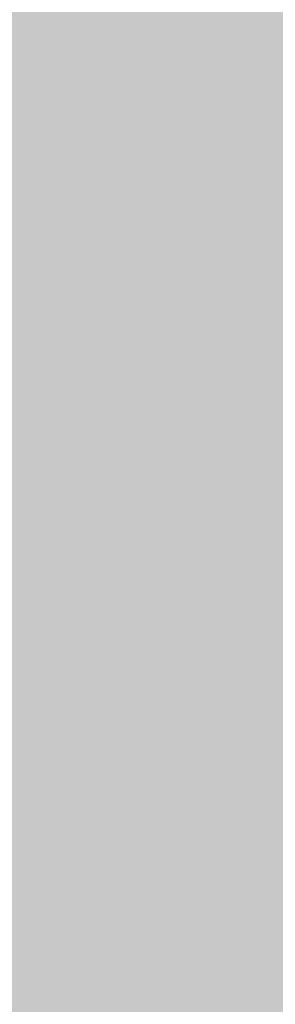
# Model space of a CAD drawing. Units: inches. Extents: x 2083 to 3317, y 1141 to 2115.
# Tile 207 of 256: x 3126.67 to 3126.939, y 1264.131 to 1265.165. Entities that reach past the tile are written whole.
import ezdxf

# ---------------------------------------------------------------- set-up
doc = ezdxf.new("R2010")
doc.units = ezdxf.units.IN
doc.layers.add('A-ANNO-DIMS', color=2, linetype='Continuous', lineweight=18)
doc.layers.add('A-WALL-PATT', color=251, linetype='Continuous', lineweight=13, true_color=0x636466)
doc.styles.get("Standard").update_dxf_attribs({"font": 'arial.ttf'})
doc.dimstyles.new('ISO-25', dxfattribs={"dimtxt": 12, "dimasz": 12, "dimexe": 1.25, "dimexo": 0.625, "dimtad": 1, "dimlunit": 3, "dimtxsty": 'Standard', "dimcen": 2.5, "dimadec": 0, "dimazin": 0, "dimtfac": 1, "dimtmove": 0, "dimatfit": 3, "dimfxl": 1, "dimarcsym": 0})

# ---------------------------------------------------------------- blocks, each defined once
blk = doc.blocks.new('*D26')
at = {"layer": 'A-ANNO-DIMS', "color": 0, "lineweight": -2, "transparency": 16777216}
for p, q in [((3088.9858, 1274.9151), (3088.9858, 1270.952)), ((3111.24, 1274.9151), (3111.24, 1270.952)), ((3076.9858, 1272.202), (2840.2624, 1272.202)), ((3111.24, 1272.202), (3088.9858, 1272.202)), ((3123.24, 1272.202), (3135.24, 1272.202))]:
    blk.add_line(p, q, dxfattribs=at)
at = {"layer": 'A-ANNO-DIMS', "color": 0, "transparency": 16777216}
for points in [[(3076.9858, 1274.202), (3076.9858, 1270.202), (3088.9858, 1272.202)], [(3123.24, 1274.202), (3123.24, 1270.202), (3111.24, 1272.202)]]:
    blk.add_solid(points, dxfattribs=at)
at = {"layer": 'Defpoints', "color": 0, "transparency": 16777216}
for p in [(3088.9858, 1275.5401), (3111.24, 1275.5401), (3088.9858, 1272.202)]:
    blk.add_point(p, dxfattribs=at)
at = {"layer": 'A-ANNO-DIMS', "color": 0, "transparency": 16777216, "insert": (2952.6241, 1279.0316), "char_height": 12, "attachment_point": 5}
blk.add_mtext('NIGHTSTAND 1\'-10 1/2" TYP.', dxfattribs=at)
blk = doc.blocks.new('*D27')
at = {"layer": 'A-ANNO-DIMS', "color": 0, "lineweight": -2, "transparency": 16777216}
for p, q in [((3114.5782, 1309.7943), (3114.5782, 1321.7943)), ((3111.865, 1297.7943), (3115.8282, 1297.7943)), ((3114.5782, 1297.7943), (3114.5782, 1275.5401)), ((3111.865, 1275.5401), (3115.8282, 1275.5401)), ((3114.5782, 1263.5401), (3114.5782, 1140.9886))]:
    blk.add_line(p, q, dxfattribs=at)
at = {"layer": 'A-ANNO-DIMS', "color": 0, "transparency": 16777216}
for points in [[(3112.5782, 1309.7943), (3116.5782, 1309.7943), (3114.5782, 1297.7943)], [(3112.5782, 1263.5401), (3116.5782, 1263.5401), (3114.5782, 1275.5401)]]:
    blk.add_solid(points, dxfattribs=at)
at = {"layer": 'Defpoints', "color": 0, "transparency": 16777216}
for p in [(3111.24, 1297.7943), (3111.24, 1275.5401), (3114.5782, 1275.5401)]:
    blk.add_point(p, dxfattribs=at)
at = {"layer": 'A-ANNO-DIMS', "color": 0, "transparency": 16777216, "insert": (3107.7485, 1196.2643), "char_height": 12, "attachment_point": 5, "rotation": 90}
blk.add_mtext('1\'-10 1/2" TYP.', dxfattribs=at)

msp = doc.modelspace()

# ---------------------------------------------------------------- hatches: boundary and pattern name
at = {"layer": 'A-WALL-PATT'}
h = msp.add_hatch(color=256, dxfattribs=at)
h.dxf.hatch_style = 1
h.paths.add_polyline_path([(3126.9598, 2020.7614), (2748.9598, 2020.7614), (2604.9598, 2020.7614), (2226.9598, 2020.7614), (2226.9598, 1702.7614), (2466.9598, 1702.7614), (2466.9598, 1582.7614), (2418.9598, 1582.7614), (2418.9598, 1477.7614), (2226.9598, 1477.7614), (2226.9598, 1263.2614), (2544.9598, 1263.2614), (2544.9598, 1411.7614), (2604.9598, 1411.7614), (2685.9598, 1411.7614), (2685.9598, 1420.7614), (2604.9598, 1420.7614), (2604.9598, 1573.7614), (2604.9598, 1702.7614), (2604.9598, 2011.7614), (2748.9598, 2011.7614), (2748.9598, 1702.7614), (2862.9598, 1702.7614), (2862.9598, 1621.7614), (2871.9598, 1621.7614), (2871.9598, 1702.7614), (2883.9598, 1702.7614), (2883.9598, 1706.9395, -0.026459), (2883.9598, 1711.7614), (2757.9598, 1711.7614), (2757.9598, 1807.7614), (2787.9598, 1807.7614), (2787.9598, 1812.2614), (2757.9598, 1812.2614), (2757.9598, 2011.7614), (2877.9598, 2011.7614), (2877.9598, 1812.2614), (2847.9598, 1812.2614), (2847.9598, 1807.7614), (2889.8357, 1807.7614), (2889.8357, 1812.2614), (2882.4598, 1812.2614), (2882.4598, 2011.7614), (3117.9598, 2011.7614), (3117.9598, 1812.2614), (2937.8357, 1812.2614), (2937.8357, 1807.7614), (2995.7098, 1807.7614), (2995.7098, 1796.1177), (3000.2098, 1796.1177), (3000.2098, 1807.7614), (3117.9598, 1807.7614), (3117.9598, 1711.7614), (3000.2098, 1711.7614), (3000.2098, 1760.1177), (2998.5727, 1760.1177, -0.020711), (2995.7098, 1760.1177), (2995.7098, 1711.7614), (2931.9598, 1711.7614), (2931.9598, 1702.7614), (3126.9598, 1702.7614)])
h.paths.add_polyline_path([(2471.4598, 2011.7614), (2471.4598, 1810.0114), (2462.7169, 1810.0114), (2462.7169, 1805.5114), (2505.9598, 1805.5114), (2505.9598, 1810.0114), (2475.9598, 1810.0114), (2475.9598, 2011.7614), (2595.9598, 2011.7614), (2595.9598, 1810.0114), (2565.9598, 1810.0114), (2565.9598, 1805.5114), (2595.9598, 1805.5114), (2595.9598, 1711.7614), (2235.9598, 1711.7614), (2235.9598, 1805.5114), (2353.7098, 1805.5114), (2353.7098, 1796.0542), (2358.2098, 1796.0542), (2358.2098, 1805.5114), (2414.7169, 1805.5114), (2414.7169, 1810.0114), (2235.9598, 1810.0114), (2235.9598, 2011.7614)], flags=16)
h.paths.add_polyline_path([(2270.2047, 1994.61), (2270.2047, 1970.61), (2246.2047, 1970.61), (2246.2047, 1994.61)], flags=0)
edge = h.paths.add_edge_path(flags=0)
edge.add_ellipse((2332.0274, 1899.7982), major_axis=(-3.043, 3.043), ratio=0.168252, start_angle=-161.3322, end_angle=-156.3071, ccw=False)
edge.add_ellipse((2333.082, 1898.7435), major_axis=(-1.0546, 1.0546), ratio=0.453532, start_angle=-123.371, end_angle=-94.1591)
edge = h.paths.add_edge_path(flags=0)
edge.add_ellipse((2332.0274, 1968.8763), major_axis=(3.043, 3.043), ratio=0.168252, start_angle=18.6678, end_angle=23.6929)
edge.add_spline(control_points=[(2332.9256, 1970.6911), (2332.2268, 1970.3361), (2330.8937, 1969.6589), (2328.4131, 1970.9321), (2327.2039, 1967.7487), (2324.7096, 1969.9556), (2322.5328, 1967.0124), (2320.0128, 1971.2958), (2317.6803, 1968.1578), (2316.0405, 1967.102), (2315.4269, 1966.8096)], knot_values=[0, 0, 0, 0, 2.267059, 4.324559, 6.685584, 8.878641, 11.121502, 14.300359, 17.755284, 19.732645, 19.732645, 19.732645, 19.732645], degree=3, periodic=0)
edge.add_ellipse((2332.0274, 1968.8763), major_axis=(3.043, 3.043), ratio=0.168252, start_angle=18.6678, end_angle=23.6929, ccw=False)
edge.add_ellipse((2333.082, 1969.9309), major_axis=(1.0546, 1.0546), ratio=0.453532, start_angle=56.629, end_angle=85.8409, ccw=False)
edge = h.paths.add_edge_path(flags=0)
edge.add_spline(control_points=[(2296.4283, 1967.9879), (2293.6278, 1965.3363), (2287.7036, 1959.7271), (2299.7439, 1949.9957), (2294.5326, 1935.6685), (2290.5732, 1920.6035), (2293.3941, 1909.9737), (2296.1854, 1904.9665)], knot_values=[0.099185, 0.099185, 0.099185, 0.099185, 0.345301, 0.619822, 0.982653, 1.386093, 1.810555, 1.810555, 1.810555, 1.810555], degree=3, periodic=0)
edge.add_spline(control_points=[(2296.1854, 1904.9665), (2297.3836, 1902.6193), (2298.001, 1901.9493), (2298.553, 1901.4682)], knot_values=[0.006246, 0.006246, 0.006246, 0.006246, 0.055476, 0.055476, 0.055476, 0.055476], degree=3, periodic=0)
edge.add_spline(control_points=[(2298.553, 1901.4682), (2297.2586, 1900.9232), (2295.2253, 1900.2321), (2293.0602, 1900.6142), (2292.1014, 1900.7884), (2292.0896, 1900.7906)], knot_values=[0.312835, 0.312835, 0.312835, 0.312835, 0.40178, 0.474987, 0.475903, 0.475903, 0.475903, 0.475903], degree=3, periodic=0)
edge.add_arc((2292.7936, 1904.6641), 3.937, 215.4209, 259.6982, ccw=False)
edge.add_spline(control_points=[(2289.5853, 1902.3823), (2289.4767, 1902.5351), (2289.3685, 1902.688), (2289.2609, 1902.8412)], knot_values=[0.102872, 0.102872, 0.102872, 0.102872, 0.116896, 0.116896, 0.116896, 0.116896], degree=3, periodic=0)
edge.add_spline(control_points=[(2289.2609, 1902.8412), (2288.6866, 1902.5502), (2287.64, 1902.0199), (2285.8813, 1901.874), (2283.853, 1901.5044), (2281.72, 1899.7105), (2278.467, 1899.4929), (2276.1571, 1901.8832), (2272.259, 1899.8041), (2267.7776, 1901.8432), (2262.2439, 1900.184), (2257.4149, 1901.7821), (2254.3184, 1900.7261), (2253.1783, 1900.3373)], knot_values=[0, 0, 0, 0, 1.907977, 3.477176, 5.261074, 7.972851, 11.680248, 13.717921, 16.939592, 22.789562, 27.502503, 33.595215, 37.145618, 37.145618, 37.145618, 37.145618], degree=3, periodic=0)
edge.add_line((2253.1783, 1900.3373), (2250.2442, 1902.8412))
edge.add_line((2250.2442, 1902.8412), (2250.2442, 1965.8333))
edge.add_line((2250.2442, 1965.8333), (2253.1783, 1968.3371))
edge.add_spline(control_points=[(2253.1783, 1968.3371), (2254.3184, 1967.9483), (2257.4149, 1966.8924), (2262.2439, 1968.4904), (2267.7776, 1966.8313), (2271.5267, 1968.5372), (2273.8759, 1967.8283), (2274.2067, 1967.7276)], knot_values=[0, 0, 0, 0, 0.09018, 0.244935, 0.364644, 0.513233, 0.537855, 0.537855, 0.537855, 0.537855], degree=3, periodic=0)
edge.add_arc((2274.3529, 1963.7933), 3.937, 72.0511, 92.1279, ccw=False)
edge.add_arc((2281.2969, 1985.23), 18.5963, 252.05113, 288.56572)
edge.add_arc((2292.3167, 1956.0289), 12.6461, 71.02679, 113.77822, ccw=False)
edge = h.paths.add_edge_path(flags=0)
edge.add_spline(control_points=[(2274.8994, 1951.8562), (2275.0662, 1951.6166), (2275.2327, 1951.3766), (2275.398, 1951.1359)], knot_values=[1.409916, 1.409916, 1.409916, 1.409916, 1.43159, 1.43159, 1.43159, 1.43159], degree=3, periodic=0)
edge.add_spline(control_points=[(2275.398, 1951.1359), (2275.7921, 1950.5619), (2276.1792, 1949.9838), (2276.5455, 1949.3971)], knot_values=[1.358238, 1.358238, 1.358238, 1.358238, 1.409916, 1.409916, 1.409916, 1.409916], degree=3, periodic=0)
edge.add_line((2276.5455, 1949.3971), (2277.4373, 1947.8622))
edge.add_spline(control_points=[(2277.4373, 1947.8622), (2276.3038, 1945.6731), (2274.6397, 1942.4269), (2274.6316, 1938.0939), (2272.7991, 1930.8515), (2274.3564, 1943.897), (2275.9477, 1947.9234), (2276.5455, 1949.3971)], knot_values=[0.005632, 0.005632, 0.005632, 0.005632, 0.186014, 0.266002, 0.357087, 0.59639, 0.739732, 0.739732, 0.739732, 0.739732], degree=3, periodic=0)
edge.add_spline(control_points=[(2276.5455, 1949.3971), (2276.1792, 1949.9838), (2275.7921, 1950.5619), (2275.398, 1951.1359)], knot_values=[1.358238, 1.358238, 1.358238, 1.358238, 1.409916, 1.409916, 1.409916, 1.409916], degree=3, periodic=0)
edge.add_spline(control_points=[(2275.398, 1951.1359), (2274.9425, 1950.0805), (2274.2078, 1948.0253), (2273.9346, 1944.8515), (2272.4685, 1937.6275), (2273.4662, 1945.6965), (2274.7006, 1951.0595), (2274.8994, 1951.8562)], knot_values=[0.104364, 0.104364, 0.104364, 0.104364, 0.189636, 0.269624, 0.36071, 0.600013, 0.644622, 0.644622, 0.644622, 0.644622], degree=3, periodic=0)
h.paths.add_polyline_path([(2269.1675, 1963.1276, -0.357527), (2268.1706, 1960.9764, -0.092561), (2268.1706, 1939.4363, -0.357527), (2269.1675, 1937.2851, -0.357527), (2267.0163, 1938.282, -0.164785), (2254.6856, 1938.282, -0.357527), (2252.5344, 1937.2851, -0.357527), (2253.5313, 1939.4363, -0.092561), (2253.5313, 1960.9764, -0.357527), (2252.5344, 1963.1276, -0.357527), (2254.6856, 1962.1307, -0.164785), (2267.0163, 1962.1307, -0.357527)], flags=0)
h.paths.add_polyline_path([(2248.8741, 1967.8018), (2248.8741, 1957.0277), (2249.4578, 1957.0277), (2249.4578, 1911.6468), (2248.8741, 1911.6468), (2248.8741, 1900.8727), (2246.5119, 1900.8727, 0.197327), (2244.1497, 1902.4569), (2244.1497, 1966.2176, 0.197327), (2246.5119, 1967.8018)], flags=0)
h.paths.add_polyline_path([(2269.1675, 1931.3893, -0.357527), (2268.1706, 1929.2381, -0.092561), (2268.1706, 1907.6981, -0.357527), (2269.1675, 1905.5469, -0.357527), (2267.0163, 1906.5438, -0.164785), (2254.6856, 1906.5438, -0.357527), (2252.5344, 1905.5469, -0.357527), (2253.5313, 1907.6981, -0.092561), (2253.5313, 1929.2381, -0.357527), (2252.5344, 1931.3893, -0.357527), (2254.6856, 1930.3925, -0.164785), (2267.0163, 1930.3925, -0.357527)], flags=0)
edge = h.paths.add_edge_path(flags=0)
edge.add_spline(control_points=[(2276.1969, 1906.7237), (2276.1681, 1909.0289), (2276.114, 1913.3719), (2270.5984, 1924.925), (2273.9052, 1919.0128), (2275.9217, 1916.2621), (2275.4746, 1912.4021), (2277.2579, 1910.3806), (2276.696, 1908.225), (2276.6462, 1906.813), (2276.6178, 1906.0084)], knot_values=[0, 0, 0, 0, 8.61026, 16.221274, 18.843057, 23.804898, 27.440828, 29.356102, 31.203478, 33.650687, 33.650687, 33.650687, 33.650687], degree=3, periodic=0)
edge.add_spline(control_points=[(2276.6178, 1906.0084), (2276.6233, 1905.6241), (2276.4977, 1904.6287), (2275.4418, 1903.8547), (2274.9373, 1903.0804), (2274.8591, 1902.8412)], knot_values=[0.156488, 0.156488, 0.156488, 0.156488, 0.184398, 0.231376, 0.250598, 0.250598, 0.250598, 0.250598], degree=3, periodic=0)
edge.add_line((2274.8591, 1902.8412), (2276.506, 1902.8412))
edge.add_spline(control_points=[(2276.506, 1902.8412), (2276.7883, 1903.0849), (2277.6651, 1904.1252), (2278.2495, 1904.3407), (2277.6539, 1908.5274), (2278.1557, 1906.2278), (2278.1005, 1905.2859), (2278.8467, 1904.069), (2277.8568, 1903.4149), (2277.8742, 1902.991), (2277.9036, 1902.8412)], knot_values=[0.059574, 0.059574, 0.059574, 0.059574, 0.080753, 0.103741, 0.16972, 0.176036, 0.207137, 0.240474, 0.262341, 0.27366, 0.27366, 0.27366, 0.27366], degree=3, periodic=0)
edge.add_line((2277.9036, 1902.8412), (2280.0298, 1902.8412))
edge.add_spline(control_points=[(2280.0298, 1902.8412), (2279.8882, 1903.0884), (2279.4993, 1903.9816), (2280.1523, 1905.9393), (2278.1036, 1909.6578), (2279.7624, 1907.1853), (2280.3279, 1904.8749), (2280.4851, 1903.4896), (2281.4633, 1903.2494), (2281.7583, 1902.9365), (2281.834, 1902.8412)], knot_values=[0.013856, 0.013856, 0.013856, 0.013856, 0.034874, 0.088867, 0.107879, 0.126738, 0.158714, 0.193757, 0.217487, 0.226722, 0.226722, 0.226722, 0.226722], degree=3, periodic=0)
edge.add_spline(control_points=[(2281.834, 1902.8412), (2281.7875, 1902.8267), (2281.647, 1902.783), (2281.3955, 1902.8595), (2281.0881, 1902.9852), (2280.7207, 1903.0609), (2280.3335, 1903.0257), (2280.1248, 1902.8989), (2280.0298, 1902.8412)], knot_values=[0, 0, 0, 0, 0.14413, 0.435517, 0.749276, 1.153046, 1.548371, 1.878348, 1.878348, 1.878348, 1.878348], degree=3, periodic=0)
edge.add_line((2280.0298, 1902.8412), (2277.9036, 1902.8412))
edge.add_spline(control_points=[(2277.9036, 1902.8412), (2277.8929, 1902.7959), (2277.8654, 1902.6796), (2277.6075, 1902.6875), (2277.2741, 1902.8007), (2276.8379, 1902.6198), (2276.5838, 1902.7893), (2276.506, 1902.8412)], knot_values=[0, 0, 0, 0, 0.127189, 0.326199, 0.628009, 1.24357, 1.515331, 1.515331, 1.515331, 1.515331], degree=3, periodic=0)
edge.add_line((2276.506, 1902.8412), (2274.8591, 1902.8412))
edge.add_spline(control_points=[(2274.8591, 1902.8412), (2274.8144, 1902.8986), (2274.7251, 1903.0134), (2274.4935, 1903.119), (2274.2443, 1902.9605), (2273.9371, 1903.1849), (2273.614, 1902.9831), (2273.4083, 1902.883), (2273.3223, 1902.8412)], knot_values=[0, 0, 0, 0, 0.21843, 0.436957, 0.687977, 0.990379, 1.398396, 1.69185, 1.69185, 1.69185, 1.69185], degree=3, periodic=0)
edge.add_spline(control_points=[(2273.3223, 1902.8412), (2273.6167, 1903.4457), (2274.274, 1904.5383), (2276.0272, 1904.5737), (2276.207, 1906.5836), (2276.1969, 1906.7237)], knot_values=[0.012227, 0.012227, 0.012227, 0.012227, 0.059472, 0.106218, 0.134458, 0.134458, 0.134458, 0.134458], degree=3, periodic=0)
h.paths.add_polyline_path([(2270.7761, 1897.7898), (2270.7761, 1873.7898), (2246.7761, 1873.7898), (2246.7761, 1897.7898)], flags=0)
h.paths.add_polyline_path([(2353.7098, 1760.0051), (2353.7098, 1760.0542), (2358.2098, 1760.0542, -0.033729)], flags=0)
h.paths.add_polyline_path([(2321.8191, 1737.5292), (2341.9953, 1737.5292, -0.414214), (2343.2033, 1736.3212), (2343.2033, 1721.0206, -0.414214), (2341.9953, 1719.8127), (2321.8191, 1719.8127, -0.414214), (2320.6112, 1721.0206), (2320.6112, 1736.3212, -0.414214)], flags=0)
h.paths.add_polyline_path([(2324.235, 1736.3212), (2339.5794, 1736.3212, -0.414214), (2341.9953, 1733.9053), (2341.9953, 1725.4497, -0.414214), (2339.5794, 1723.0338), (2333.6806, 1723.0338), (2333.8453, 1722.0455, -0.870646), (2335.4254, 1721.8259, -0.767327), (2333.9227, 1721.4232), (2331.291, 1721.4232, -0.767327), (2329.7883, 1721.8259, -0.870646), (2331.3684, 1722.0455), (2331.5331, 1723.0338), (2324.235, 1723.0338, -0.414214), (2321.8191, 1725.4497), (2321.8191, 1733.9053, -0.414214)], flags=0)
h.paths.add_polyline_path([(2570.4838, 1928.6154), (2589.6838, 1928.6154), (2590.1688, 1928.6154), (2590.1688, 1904.9934), (2570.4838, 1904.9934)], flags=0)
h.paths.add_polyline_path([(2574.4473, 1927.2638, -1), (2572.8288, 1927.2638, -1)], flags=0)
h.paths.add_polyline_path([(2573.0899, 1926.9409), (2573.925, 1927.776), (2574.1477, 1927.5533), (2573.3126, 1926.7182)], flags=0)
h.paths.add_polyline_path([(2578.7791, 1919.7296, -1), (2571.5917, 1919.7296, -1)], flags=0)
h.paths.add_polyline_path([(2578.3854, 1919.7296, -1), (2571.9854, 1919.7296, -1)], flags=0)
h.paths.add_polyline_path([(2331.5958, 1729.4762, -1), (2333.618, 1729.4762, -1)], flags=0)
h.paths.add_polyline_path([(2578.0342, 1927.2638, -1), (2576.4157, 1927.2638, -1)], flags=0)
h.paths.add_polyline_path([(2576.6889, 1927.5311), (2576.9116, 1927.7538), (2577.7467, 1926.9186), (2577.524, 1926.6959)], flags=0)
h.paths.add_polyline_path([(2578.1391, 1909.8595, -1), (2572.2317, 1909.8595, -1)], flags=0)
h.paths.add_polyline_path([(2577.7454, 1909.8595, -1), (2572.6254, 1909.8595, -1)], flags=0)
h.paths.add_polyline_path([(2583.7977, 1927.2638, -1), (2582.1792, 1927.2638, -1)], flags=0)
h.paths.add_polyline_path([(2582.7186, 1927.7538), (2583.5538, 1926.9186), (2583.3311, 1926.6959), (2582.4959, 1927.5311)], flags=0)
h.paths.add_polyline_path([(2582.4959, 1927.5311), (2582.7186, 1927.7538), (2583.5538, 1926.9186), (2583.3311, 1926.6959)], flags=0)
h.paths.add_polyline_path([(2587.7391, 1920.5296, -1), (2581.8317, 1920.5296, -1)], flags=0)
h.paths.add_polyline_path([(2587.3454, 1920.5296, -1), (2582.2254, 1920.5296, -1)], flags=0)
h.paths.add_polyline_path([(2587.3846, 1927.2638, -1), (2585.7661, 1927.2638, -1)], flags=0)
h.paths.add_polyline_path([(2586.082, 1926.9802), (2586.9172, 1927.8154), (2587.1399, 1927.5927), (2586.3047, 1926.7575)], flags=0)
h.paths.add_polyline_path([(2588.3791, 1910.6595, -1), (2581.1917, 1910.6595, -1)], flags=0)
h.paths.add_polyline_path([(2587.9854, 1910.6595, -1), (2581.5854, 1910.6595, -1)], flags=0)
h.paths.add_polyline_path([(2417.1677, 1729.4779), (2437.3439, 1729.4779, -0.414214), (2438.5519, 1728.2699), (2438.5519, 1712.9693, -0.414214), (2437.3439, 1711.7614), (2417.1677, 1711.7614, -0.414214), (2415.9598, 1712.9693), (2415.9598, 1728.2699, -0.414214)], flags=0)
h.paths.add_polyline_path([(2419.5836, 1728.2699), (2434.928, 1728.2699, -0.414214), (2437.3439, 1725.8541), (2437.3439, 1717.3984, -0.414214), (2434.928, 1714.9825), (2429.0292, 1714.9825), (2429.1939, 1713.9942, -0.870646), (2430.774, 1713.7746, -0.767327), (2429.2713, 1713.372), (2426.6396, 1713.372, -0.767327), (2425.1369, 1713.7746, -0.870646), (2426.717, 1713.9942), (2426.8817, 1714.9825), (2419.5836, 1714.9825, -0.414214), (2417.1677, 1717.3984), (2417.1677, 1725.8541, -0.414214)], flags=0)
h.paths.add_polyline_path([(2419.5836, 1728.2699), (2434.928, 1728.2699, -0.414214), (2437.3439, 1725.8541), (2437.3439, 1717.3984, -0.414214), (2434.928, 1714.9825), (2429.0292, 1714.9825), (2428.3581, 1719.009), (2427.5528, 1719.009), (2426.8817, 1714.9825), (2419.5836, 1714.9825, -0.414214), (2417.1677, 1717.3984), (2417.1677, 1725.8541, -0.414214)], flags=0)
h.paths.add_polyline_path([(2426.9444, 1721.4249, -1), (2428.9666, 1721.4249, -1)], flags=0)
h.paths.add_polyline_path([(2475.9598, 1702.7614), (2595.9598, 1702.7614), (2595.9598, 1582.7614), (2475.9598, 1582.7614)], flags=16)
h.paths.add_polyline_path([(2427.9598, 1573.7614), (2595.9598, 1573.7614), (2595.9598, 1468.7614), (2595.9598, 1420.7614), (2384.4598, 1420.7614), (2384.4598, 1468.7614), (2427.9598, 1468.7614)], flags=16)
h.paths.add_polyline_path([(2379.9598, 1468.7614), (2379.9598, 1420.7614), (2235.9598, 1420.7614), (2235.9598, 1468.7614)], flags=16)
h.paths.add_polyline_path([(2317.816, 1466.6958), (2337.9922, 1466.6958, -0.414214), (2339.2002, 1465.4878), (2339.2002, 1450.1872, -0.414214), (2337.9922, 1448.9792), (2317.816, 1448.9792, -0.414214), (2316.6081, 1450.1872), (2316.6081, 1465.4878, -0.414214)], flags=0)
h.paths.add_polyline_path([(2320.2319, 1465.4878), (2335.5763, 1465.4878, -0.414214), (2337.9922, 1463.0719), (2337.9922, 1454.6163, -0.414214), (2335.5763, 1452.2004), (2329.6775, 1452.2004), (2329.8422, 1451.212, -0.870646), (2331.4223, 1450.9925, -0.767327), (2329.9196, 1450.5898), (2327.2879, 1450.5898, -0.767327), (2325.7852, 1450.9925, -0.870646), (2327.3653, 1451.212), (2327.53, 1452.2004), (2320.2319, 1452.2004, -0.414214), (2317.816, 1454.6163), (2317.816, 1463.0719, -0.414214)], flags=0)
h.paths.add_polyline_path([(2320.2319, 1465.4878), (2335.5763, 1465.4878, -0.414214), (2337.9922, 1463.0719), (2337.9922, 1454.6163, -0.414214), (2335.5763, 1452.2004), (2329.6775, 1452.2004), (2329.0064, 1456.2269), (2328.2011, 1456.2269), (2327.53, 1452.2004), (2320.2319, 1452.2004, -0.414214), (2317.816, 1454.6163), (2317.816, 1463.0719, -0.414214)], flags=0)
h.paths.add_polyline_path([(2327.5926, 1458.6428, -1), (2329.6148, 1458.6428, -1)], flags=0)
h.paths.add_polyline_path([(2244.4117, 1433.3405), (2241.9209, 1433.3405, -0.414214), (2240.0179, 1435.2435), (2240.0179, 1440.9528, -0.414211), (2241.9209, 1442.8559), (2244.4117, 1442.8559, -1.976472)], flags=0)
h.paths.add_polyline_path([(2245.3569, 1434.3975, -0.414214), (2245.3569, 1441.7988, -2.144098)], flags=0)
h.paths.add_polyline_path([(2535.9598, 1416.2614), (2535.9598, 1272.2614), (2235.9598, 1272.2614), (2235.9598, 1416.2614)], flags=16)
h.paths.add_polyline_path([(2260.1196, 1384.2928), (2260.1196, 1362.0386), (2237.8654, 1362.0386), (2237.8654, 1384.2928)], flags=0)
edge = h.paths.add_edge_path(flags=0)
edge.add_line((2318.2518, 1362.0933), (2318.1458, 1362.001))
edge.add_ellipse((2317.4451, 1360.431), major_axis=(2.8216, 2.8216), ratio=0.168252, start_angle=18.6678, end_angle=20.9481, ccw=False)
edge.add_ellipse((2318.423, 1361.409), major_axis=(0.9779, 0.9779), ratio=0.453532, start_angle=56.629, end_angle=70.2262, ccw=False)
edge = h.paths.add_edge_path(flags=0)
edge.add_line((2319.1074, 1295.5711), (2319.015, 1295.6771))
edge.add_ellipse((2317.4451, 1296.3778), major_axis=(-2.8216, 2.8216), ratio=0.168252, start_angle=-161.3322, end_angle=-159.0519, ccw=False)
edge.add_ellipse((2318.423, 1295.3999), major_axis=(-0.9779, 0.9779), ratio=0.453532, start_angle=-123.371, end_angle=-109.7738)
edge = h.paths.add_edge_path(flags=0)
edge.add_spline(control_points=[(2284.2103, 1301.1702), (2284.5807, 1300.4447), (2284.8912, 1299.892), (2285.1596, 1299.461)], knot_values=[0.039066, 0.039066, 0.039066, 0.039066, 0.055476, 0.055476, 0.055476, 0.055476], degree=3, periodic=0)
edge.add_line((2285.1596, 1299.461), (2284.2103, 1301.1702))
edge = h.paths.add_edge_path(flags=0)
edge.add_line((2280.4125, 1297.298), (2283.37, 1297.0361))
edge.add_line((2283.37, 1297.0361), (2286.4057, 1297.9263))
edge.add_spline(control_points=[(2286.4057, 1297.9263), (2285.3055, 1297.4631), (2284.3448, 1297.1292), (2283.37, 1297.0361)], knot_values=[0.394369, 0.394369, 0.394369, 0.394369, 0.475903, 0.475903, 0.475903, 0.475903], degree=3, periodic=0)
edge.add_spline(control_points=[(2283.37, 1297.0361), (2283.2814, 1297.0277), (2282.3163, 1296.9573), (2281.3125, 1297.1345), (2280.4234, 1297.296), (2280.4125, 1297.298)], knot_values=[0.312835, 0.312835, 0.312835, 0.312835, 0.320246, 0.393453, 0.394369, 0.394369, 0.394369, 0.394369], degree=3, periodic=0)
edge = h.paths.add_edge_path(flags=0)
edge.add_line((2284.4356, 1359.6073), (2280.4463, 1355.328))
edge.add_line((2280.4463, 1355.328), (2279.58, 1351.0178))
edge.add_line((2279.58, 1351.0178), (2282.413, 1346.5804))
edge.add_spline(control_points=[(2282.413, 1346.5804), (2283.1533, 1345.5892), (2284.2529, 1344.0289), (2284.801, 1342.3872), (2284.9352, 1341.8055)], knot_values=[1.240098, 1.240098, 1.240098, 1.240098, 1.332892, 1.382712, 1.382712, 1.382712, 1.382712], degree=3, periodic=0)
edge.add_spline(control_points=[(2284.9352, 1341.8055), (2285.3191, 1340.1406), (2285.233, 1338.4092), (2284.9099, 1336.6541)], knot_values=[1.097484, 1.097484, 1.097484, 1.097484, 1.240098, 1.240098, 1.240098, 1.240098], degree=3, periodic=0)
edge.add_spline(control_points=[(2284.9099, 1336.6541), (2284.5868, 1334.899), (2284.0267, 1333.1203), (2283.4626, 1331.3606)], knot_values=[0.95487, 0.95487, 0.95487, 0.95487, 1.097484, 1.097484, 1.097484, 1.097484], degree=3, periodic=0)
edge.add_line((2283.4626, 1331.3606), (2281.8904, 1326.1534))
edge.add_line((2281.8904, 1326.1534), (2280.7563, 1321.0561))
edge.add_line((2280.7563, 1321.0561), (2280.2992, 1316.002))
edge.add_line((2280.2992, 1316.002), (2280.7159, 1310.9501))
edge.add_line((2280.7159, 1310.9501), (2282.0281, 1305.9721))
edge.add_line((2282.0281, 1305.9721), (2284.2103, 1301.1702))
edge.add_spline(control_points=[(2284.2103, 1301.1702), (2283.3407, 1302.7302), (2282.6119, 1304.3365), (2282.0281, 1305.9721)], knot_values=[0.099185, 0.099185, 0.099185, 0.099185, 0.241799, 0.241799, 0.241799, 0.241799], degree=3, periodic=0)
edge.add_spline(control_points=[(2282.0281, 1305.9721), (2281.4443, 1307.6078), (2281.0055, 1309.2728), (2280.7159, 1310.9501)], knot_values=[0.241799, 0.241799, 0.241799, 0.241799, 0.384413, 0.384413, 0.384413, 0.384413], degree=3, periodic=0)
edge.add_spline(control_points=[(2280.7159, 1310.9501), (2280.4332, 1312.5876), (2280.2894, 1314.277), (2280.2989, 1315.962), (2280.2992, 1316.002)], knot_values=[0.384413, 0.384413, 0.384413, 0.384413, 0.523647, 0.527028, 0.527028, 0.527028, 0.527028], degree=3, periodic=0)
edge.add_spline(control_points=[(2280.2992, 1316.002), (2280.3123, 1317.687), (2280.4779, 1319.3679), (2280.7563, 1321.0561)], knot_values=[0.527028, 0.527028, 0.527028, 0.527028, 0.669642, 0.669642, 0.669642, 0.669642], degree=3, periodic=0)
edge.add_spline(control_points=[(2280.7563, 1321.0561), (2281.0346, 1322.7443), (2281.4259, 1324.4396), (2281.8904, 1326.1534)], knot_values=[0.669642, 0.669642, 0.669642, 0.669642, 0.812256, 0.812256, 0.812256, 0.812256], degree=3, periodic=0)
edge.add_spline(control_points=[(2281.8904, 1326.1534), (2282.2644, 1327.5333), (2282.7879, 1329.2618), (2283.3528, 1331.0178), (2283.4626, 1331.3606)], knot_values=[0.812256, 0.812256, 0.812256, 0.812256, 0.927087, 0.95487, 0.95487, 0.95487, 0.95487], degree=3, periodic=0)
edge.add_line((2283.4626, 1331.3606), (2284.9099, 1336.6541))
edge.add_line((2284.9099, 1336.6541), (2284.9352, 1341.8055))
edge.add_line((2284.9352, 1341.8055), (2282.413, 1346.5804))
edge.add_spline(control_points=[(2282.413, 1346.5804), (2281.2751, 1348.1038), (2280.0784, 1349.5703), (2279.58, 1351.0178)], knot_values=[1.382712, 1.382712, 1.382712, 1.382712, 1.525326, 1.525326, 1.525326, 1.525326], degree=3, periodic=0)
edge.add_spline(control_points=[(2279.58, 1351.0178), (2279.4433, 1351.4147), (2279.1363, 1352.8569), (2279.7352, 1354.2904), (2280.4463, 1355.328)], knot_values=[1.525326, 1.525326, 1.525326, 1.525326, 1.564439, 1.667941, 1.667941, 1.667941, 1.667941], degree=3, periodic=0)
edge.add_spline(control_points=[(2280.4463, 1355.328), (2281.4261, 1356.7578), (2282.9308, 1358.1826), (2284.4356, 1359.6073)], knot_values=[1.667941, 1.667941, 1.667941, 1.667941, 1.810555, 1.810555, 1.810555, 1.810555], degree=3, periodic=0)
edge.add_arc((2280.6231, 1348.5182), 11.7262, 71.02679, 113.77822)
edge.add_arc((2270.4049, 1375.5952), 17.2436, 252.05113, 288.56572, ccw=False)
edge.add_arc((2263.966, 1355.7178), 3.6506, 72.0511, 92.1279)
edge.add_arc((2263.966, 1355.7178), 3.6506, 92.1279, 177.9851)
edge.add_spline(control_points=[(2260.3176, 1355.8462), (2260.2604, 1354.2207), (2260.5513, 1350.1865), (2262.9993, 1346.7663), (2264.4727, 1344.649)], knot_values=[1.43159, 1.43159, 1.43159, 1.43159, 1.564144, 1.770695, 1.770695, 1.770695, 1.770695], degree=3, periodic=0)
edge.add_line((2264.4727, 1344.649), (2264.9356, 1343.9825))
edge.add_spline(control_points=[(2263.801, 1340.2481), (2263.8432, 1340.5141), (2264.0672, 1341.7565), (2264.5127, 1343.0025), (2264.935, 1343.9811)], knot_values=[0.53657, 0.53657, 0.53657, 0.53657, 0.559349, 0.644622, 0.644622, 0.644622, 0.644622], degree=3, periodic=0)
edge.add_spline(control_points=[(2264.935, 1343.9811), (2265.1178, 1343.715), (2265.2989, 1343.4479), (2265.4768, 1343.1794)], knot_values=[1.384077, 1.384077, 1.384077, 1.384077, 1.409916, 1.409916, 1.409916, 1.409916], degree=3, periodic=0)
edge.add_spline(control_points=[(2265.4768, 1343.1794), (2265.6546, 1342.9108), (2265.8293, 1342.6408), (2265.9991, 1342.3688)], knot_values=[1.358238, 1.358238, 1.358238, 1.358238, 1.384077, 1.384077, 1.384077, 1.384077], degree=3, periodic=0)
edge.add_line((2265.9991, 1342.3688), (2266.826, 1340.9455))
edge.add_spline(control_points=[(2266.826, 1340.9455), (2268.8944, 1337.0897), (2271.3982, 1325.843), (2270.5162, 1310.5686), (2275.9194, 1301.8606), (2277.7895, 1299.1994)], knot_values=[0.116896, 0.116896, 0.116896, 0.116896, 0.472987, 1.050969, 1.313793, 1.313793, 1.313793, 1.313793], degree=3, periodic=0)
edge.add_spline(control_points=[(2277.7895, 1299.1994), (2277.8394, 1299.1285), (2277.8894, 1299.0575), (2277.9396, 1298.9866)], knot_values=[0.109884, 0.109884, 0.109884, 0.109884, 0.116896, 0.116896, 0.116896, 0.116896], degree=3, periodic=0)
edge.add_line((2277.9396, 1298.9866), (2277.7888, 1299.1991))
edge.add_spline(control_points=[(2277.7888, 1299.1991), (2277.2566, 1298.9294), (2276.2864, 1298.4379), (2275.0394, 1298.3344), (2274.3833, 1298.2389), (2274.2153, 1298.2093)], knot_values=[33.12187, 33.12187, 33.12187, 33.12187, 35.029056, 36.598255, 37.144827, 37.144827, 37.144827, 37.144827], degree=3, periodic=0)
edge.add_line((2274.2153, 1298.2093), (2273.0731, 1297.893))
edge.add_spline(control_points=[(2273.0731, 1297.893), (2272.3229, 1297.5798), (2271.0392, 1296.5105), (2269.2484, 1296.2261), (2268.4231, 1296.3747)], knot_values=[26.532584, 26.532584, 26.532584, 26.532584, 29.198919, 31.839101, 31.839101, 31.839101, 31.839101], degree=3, periodic=0)
edge.add_line((2268.4231, 1296.3747), (2263.8785, 1297.4575))
edge.add_spline(control_points=[(2263.8785, 1297.4575), (2263.5561, 1297.3594), (2261.8603, 1296.8387), (2260.2388, 1297.2824), (2258.9335, 1297.5165)], knot_values=[15.919551, 15.919551, 15.919551, 15.919551, 16.939592, 21.226067, 21.226067, 21.226067, 21.226067], degree=3, periodic=0)
edge.add_line((2258.9335, 1297.5165), (2254.0552, 1297.329))
edge.add_spline(control_points=[(2254.0552, 1297.329), (2253.7555, 1297.2958), (2252.1137, 1297.1652), (2250.4619, 1297.5442), (2249.1297, 1297.6679)], knot_values=[5.306517, 5.306517, 5.306517, 5.306517, 6.276435, 10.613034, 10.613034, 10.613034, 10.613034], degree=3, periodic=0)
edge.add_line((2249.1297, 1297.6679), (2244.3316, 1296.8778))
edge.add_line((2244.3316, 1296.8778), (2241.611, 1299.1994))
edge.add_line((2241.611, 1299.1994), (2241.611, 1357.6094))
edge.add_line((2241.611, 1357.6094), (2244.3316, 1359.9311))
edge.add_line((2244.3316, 1359.9311), (2252.7288, 1359.5427))
edge.add_spline(control_points=[(2252.7288, 1359.5427), (2252.8709, 1359.5464), (2253.3057, 1359.5482), (2253.7398, 1359.5143), (2254.0317, 1359.4824)], knot_values=[0.233291, 0.233291, 0.233291, 0.233291, 0.244935, 0.268927, 0.268927, 0.268927, 0.268927], degree=3, periodic=0)
edge.add_line((2254.0317, 1359.4824), (2259.5872, 1359.4164))
edge.add_spline(control_points=[(2259.5872, 1359.4164), (2260.6771, 1359.6285), (2262.0732, 1359.897), (2263.5237, 1359.4593), (2263.8304, 1359.366)], knot_values=[0.422516, 0.422516, 0.422516, 0.422516, 0.513233, 0.537855, 0.537855, 0.537855, 0.537855], degree=3, periodic=0)
edge.add_arc((2263.966, 1355.7178), 3.6506, 72.0511, 92.1279, ccw=False)
edge.add_arc((2270.4049, 1375.5952), 17.2436, 252.05113, 288.56572)
edge.add_arc((2280.6231, 1348.5182), 11.7262, 71.02679, 113.77822, ccw=False)
h.paths.add_polyline_path([(2240.3405, 1359.4347), (2240.3405, 1349.4444), (2240.8818, 1349.4444), (2240.8818, 1307.3645), (2240.3405, 1307.3645), (2240.3405, 1297.3741), (2238.1502, 1297.3741, 0.197327), (2235.9598, 1298.8431), (2235.9598, 1357.9657, 0.197327), (2238.1502, 1359.4347)], flags=0)
h.paths.add_polyline_path([(2259.1578, 1355.1005, -0.357527), (2258.2334, 1353.1058, -0.092561), (2258.2334, 1333.1326, -0.357527), (2259.1578, 1331.1379, -0.357527), (2257.1631, 1332.0622, -0.164785), (2245.7293, 1332.0622, -0.357527), (2243.7346, 1331.1379, -0.357527), (2244.6589, 1333.1326, -0.092561), (2244.6589, 1353.1058, -0.357527), (2243.7346, 1355.1005, -0.357527), (2245.7293, 1354.1761, -0.164785), (2257.1631, 1354.1761, -0.357527)], flags=0)
edge = h.paths.add_edge_path(flags=0)
edge.add_line((2265.9991, 1342.3688), (2266.826, 1340.9455))
edge.add_line((2266.826, 1340.9455), (2265.3076, 1337.8141))
edge.add_line((2265.3076, 1337.8141), (2264.3582, 1334.6529))
edge.add_line((2264.3582, 1334.6529), (2264.262, 1333.7997))
edge.add_spline(control_points=[(2264.262, 1333.7997), (2264.2084, 1333.1871), (2264.1621, 1332.3655), (2264.0071, 1331.4139), (2263.969, 1331.2018)], knot_values=[0.464444, 0.464444, 0.464444, 0.464444, 0.516691, 0.531608, 0.531608, 0.531608, 0.531608], degree=3, periodic=0)
edge.add_spline(control_points=[(2263.969, 1331.2018), (2263.7745, 1330.1189), (2263.4244, 1328.7908), (2263.2574, 1328.5307), (2263.234, 1328.5146)], knot_values=[0.372682, 0.372682, 0.372682, 0.372682, 0.44885, 0.464444, 0.464444, 0.464444, 0.464444], degree=3, periodic=0)
edge.add_spline(control_points=[(2263.234, 1328.5146), (2263.0964, 1328.4202), (2263.1312, 1329.3015), (2263.275, 1330.6157)], knot_values=[0.280919, 0.280919, 0.280919, 0.280919, 0.372682, 0.372682, 0.372682, 0.372682], degree=3, periodic=0)
edge.add_spline(control_points=[(2263.275, 1330.6157), (2263.4187, 1331.93), (2263.6715, 1333.6773), (2263.9699, 1335.315)], knot_values=[0.189157, 0.189157, 0.189157, 0.189157, 0.280919, 0.280919, 0.280919, 0.280919], degree=3, periodic=0)
edge.add_spline(control_points=[(2263.9699, 1335.315), (2264.1005, 1336.0322), (2264.4188, 1337.6219), (2264.7548, 1338.8644), (2264.9474, 1339.4911)], knot_values=[0.097394, 0.097394, 0.097394, 0.097394, 0.137578, 0.189157, 0.189157, 0.189157, 0.189157], degree=3, periodic=0)
edge.add_spline(control_points=[(2264.9474, 1339.4911), (2265.29, 1340.6061), (2265.6442, 1341.494), (2265.9991, 1342.3688)], knot_values=[0.005632, 0.005632, 0.005632, 0.005632, 0.097394, 0.097394, 0.097394, 0.097394], degree=3, periodic=0)
h.paths.add_polyline_path([(2259.1578, 1325.671, -0.357527), (2258.2334, 1323.6763, -0.092561), (2258.2334, 1303.7031, -0.357527), (2259.1578, 1301.7084, -0.357527), (2257.1631, 1302.6327, -0.164785), (2245.7293, 1302.6327, -0.357527), (2243.7346, 1301.7084, -0.357527), (2244.6589, 1303.7031, -0.092561), (2244.6589, 1323.6763, -0.357527), (2243.7346, 1325.671, -0.357527), (2245.7293, 1324.7466, -0.164785), (2257.1631, 1324.7466, -0.357527)], flags=0)
edge = h.paths.add_edge_path(flags=0)
edge.add_spline(control_points=[(2261.7089, 1317.3114), (2261.6795, 1317.4176), (2261.7619, 1317.3885), (2262.4907, 1316.0899), (2262.9622, 1315.3009)], knot_values=[14.955861, 14.955861, 14.955861, 14.955861, 16.221274, 18.694826, 18.694826, 18.694826, 18.694826], degree=3, periodic=0)
edge.add_spline(control_points=[(2262.9622, 1315.3009), (2262.9904, 1315.2536), (2263.7021, 1314.0674), (2264.349, 1313.1272), (2264.7301, 1312.1642)], knot_values=[18.694826, 18.694826, 18.694826, 18.694826, 18.843057, 22.433791, 22.433791, 22.433791, 22.433791], degree=3, periodic=0)
edge.add_spline(control_points=[(2264.7301, 1312.1642), (2264.8756, 1311.7964), (2265.1769, 1310.7698), (2265.1431, 1309.5593), (2265.2477, 1308.8242)], knot_values=[22.433791, 22.433791, 22.433791, 22.433791, 23.804898, 26.172756, 26.172756, 26.172756, 26.172756], degree=3, periodic=0)
edge.add_line((2265.2477, 1308.8242), (2265.8508, 1307.1719))
edge.add_spline(control_points=[(2265.8508, 1307.1719), (2266.065, 1306.8217), (2266.3844, 1306.3322), (2266.4244, 1305.7805), (2266.4204, 1305.6112)], knot_values=[28.062562, 28.062562, 28.062562, 28.062562, 29.356102, 29.911721, 29.911721, 29.911721, 29.911721], degree=3, periodic=0)
edge.add_spline(control_points=[(2266.4204, 1305.6112), (2266.4161, 1305.4326), (2266.394, 1305.25), (2266.3648, 1305.0659)], knot_values=[29.911721, 29.911721, 29.911721, 29.911721, 30.497837, 30.497837, 30.497837, 30.497837], degree=3, periodic=0)
edge.add_line((2266.3648, 1305.0659), (2266.0662, 1302.1363))
edge.add_spline(control_points=[(2266.0662, 1302.1363), (2266.0712, 1301.78), (2265.9981, 1301.2), (2265.6633, 1300.759), (2265.5089, 1300.5859)], knot_values=[0.156488, 0.156488, 0.156488, 0.156488, 0.184398, 0.203543, 0.203543, 0.203543, 0.203543], degree=3, periodic=0)
edge.add_line((2265.5089, 1300.5859), (2264.4353, 1299.1994))
edge.add_line((2264.4353, 1299.1994), (2265.9624, 1299.1994))
edge.add_line((2265.9624, 1299.1994), (2267.336, 1301.1753))
edge.add_line((2267.336, 1301.1753), (2267.3117, 1301.9862))
edge.add_spline(control_points=[(2267.3117, 1301.9862), (2267.2611, 1302.8624), (2267.1602, 1303.7371), (2267.2715, 1303.3259)], knot_values=[0.126229, 0.126229, 0.126229, 0.126229, 0.166617, 0.166617, 0.166617, 0.166617], degree=3, periodic=0)
edge.add_spline(control_points=[(2267.2715, 1303.3259), (2267.28, 1303.2943), (2267.3098, 1303.1754), (2267.3735, 1302.8836), (2267.4061, 1302.6828), (2267.4179, 1302.601)], knot_values=[0.166617, 0.166617, 0.166617, 0.166617, 0.16972, 0.176036, 0.180765, 0.180765, 0.180765, 0.180765], degree=3, periodic=0)
edge.add_spline(control_points=[(2267.7439, 1300.9875), (2267.6876, 1301.1509), (2267.4805, 1301.6567), (2267.4838, 1302.1448), (2267.4179, 1302.601)], knot_values=[0.180765, 0.180765, 0.180765, 0.180765, 0.193767, 0.220139, 0.220139, 0.220139, 0.220139], degree=3, periodic=0)
edge.add_line((2267.4179, 1302.601), (2267.7439, 1300.9875))
edge.add_spline(control_points=[(2267.7439, 1300.9875), (2267.832, 1300.7319), (2267.932, 1300.3099), (2267.5548, 1299.9745), (2267.4294, 1299.8292)], knot_values=[0.220139, 0.220139, 0.220139, 0.220139, 0.240474, 0.25489, 0.25489, 0.25489, 0.25489], degree=3, periodic=0)
edge.add_line((2267.4294, 1299.8292), (2267.2584, 1299.1994))
edge.add_line((2267.2584, 1299.1994), (2269.23, 1299.1994))
edge.add_spline(control_points=[(2269.23, 1299.1994), (2269.0987, 1299.4287), (2268.8428, 1300.0163), (2269.0116, 1300.9159), (2268.9468, 1301.6607)], knot_values=[0.013856, 0.013856, 0.013856, 0.013856, 0.034874, 0.067073, 0.067073, 0.067073, 0.067073], degree=3, periodic=0)
edge.add_line((2268.9468, 1301.6607), (2268.4316, 1303.6031))
edge.add_spline(control_points=[(2268.4316, 1303.6031), (2268.1756, 1304.1924), (2267.5962, 1305.2513), (2268.0407, 1304.6232), (2268.2514, 1304.2824)], knot_values=[0.090155, 0.090155, 0.090155, 0.090155, 0.107879, 0.120289, 0.120289, 0.120289, 0.120289], degree=3, periodic=0)
edge.add_spline(control_points=[(2268.2514, 1304.2824), (2268.3609, 1304.1053), (2269.0578, 1302.918), (2269.3827, 1301.5904), (2269.5214, 1300.7759), (2269.5752, 1300.5558)], knot_values=[0.120289, 0.120289, 0.120289, 0.120289, 0.126738, 0.158714, 0.173506, 0.173506, 0.173506, 0.173506], degree=3, periodic=0)
edge.add_line((2269.5752, 1300.5558), (2270.6858, 1299.4213))
edge.add_spline(control_points=[(2270.6858, 1299.4213), (2270.7672, 1299.3573), (2270.8379, 1299.2814), (2270.9029, 1299.1994)], knot_values=[0.21816, 0.21816, 0.21816, 0.21816, 0.226722, 0.226722, 0.226722, 0.226722], degree=3, periodic=0)
edge.add_line((2270.9372, 1299.1929), (2270.9029, 1299.1994))
edge.add_spline(control_points=[(2270.9029, 1299.1994), (2270.8598, 1299.186), (2270.7295, 1299.1455), (2270.4963, 1299.2164), (2270.2717, 1299.3083), (2270.121, 1299.348), (2270.0633, 1299.3596)], knot_values=[0.939174, 0.939174, 0.939174, 0.939174, 1.083304, 1.374691, 1.68845, 1.878348, 1.878348, 1.878348, 1.878348], degree=3, periodic=0)
edge.add_line((2270.0633, 1299.3596), (2269.23, 1299.1994))
edge.add_line((2269.23, 1299.1994), (2267.2584, 1299.1994))
edge.add_spline(control_points=[(2267.2584, 1299.1994), (2267.2484, 1299.1574), (2267.223, 1299.0497), (2266.9838, 1299.0569), (2266.8092, 1299.1162), (2266.6769, 1299.1091), (2266.6365, 1299.1048)], knot_values=[0.757665, 0.757665, 0.757665, 0.757665, 0.884854, 1.083864, 1.385675, 1.515331, 1.515331, 1.515331, 1.515331], degree=3, periodic=0)
edge.add_spline(control_points=[(2266.6365, 1299.1048), (2266.4852, 1299.0888), (2266.2358, 1299.0171), (2266.0346, 1299.1513), (2265.9624, 1299.1994)], knot_values=[0, 0, 0, 0, 0.485905, 0.757665, 0.757665, 0.757665, 0.757665], degree=3, periodic=0)
edge.add_line((2265.9624, 1299.1994), (2264.4353, 1299.1994))
edge.add_line((2264.4353, 1299.1994), (2263.8584, 1299.3671))
edge.add_spline(control_points=[(2263.8584, 1299.3671), (2263.8189, 1299.3709), (2263.7795, 1299.3857), (2263.7401, 1299.4015)], knot_values=[0.845925, 0.845925, 0.845925, 0.845925, 0.978627, 0.978627, 0.978627, 0.978627], degree=3, periodic=0)
edge.add_line((2263.7218, 1299.3964), (2263.0103, 1299.1994))
edge.add_spline(control_points=[(2263.0103, 1299.1994), (2263.2458, 1299.6829), (2263.506, 1300.1281), (2263.8735, 1300.408)], knot_values=[0.012227, 0.012227, 0.012227, 0.012227, 0.052971, 0.052971, 0.052971, 0.052971], degree=3, periodic=0)
edge.add_spline(control_points=[(2263.8735, 1300.408), (2263.9321, 1300.4527), (2264.0842, 1300.553), (2264.2552, 1300.6242), (2264.3597, 1300.6647)], knot_values=[0.052971, 0.052971, 0.052971, 0.052971, 0.059472, 0.069086, 0.069086, 0.069086, 0.069086], degree=3, periodic=0)
edge.add_line((2264.3597, 1300.6647), (2265.1419, 1301.0778))
edge.add_line((2265.1419, 1301.0778), (2265.6758, 1302.7996))
edge.add_line((2265.6758, 1302.7996), (2265.5407, 1305.7041))
edge.add_line((2265.5407, 1305.7041), (2264.8031, 1309.3277))
edge.add_line((2264.8031, 1309.3277), (2263.0405, 1314.0918))
edge.add_spline(control_points=[(2263.0405, 1314.0918), (2262.3836, 1315.6714), (2261.796, 1316.9977), (2261.7089, 1317.3114)], knot_values=[11.216896, 11.216896, 11.216896, 11.216896, 14.955861, 14.955861, 14.955861, 14.955861], degree=3, periodic=0)
h.paths.add_polyline_path([(2871.9598, 1416.2614), (2895.91, 1416.2614), (2895.91, 1420.7614), (2871.9598, 1420.7614), (2871.9598, 1501.7614), (2862.9598, 1501.7614), (2862.9598, 1420.7614), (2805.9598, 1420.7614), (2805.9598, 1411.7614), (2862.9598, 1411.7614), (2862.9598, 1263.2614), (3126.9598, 1263.2614), (3126.9598, 1411.7614), (3126.9598, 1486.7614), (2943.9598, 1486.7614), (2943.9598, 1477.7614), (2967.8603, 1477.7614), (2967.8603, 1420.7614), (2943.91, 1420.7614), (2943.91, 1416.2614), (3117.9598, 1416.2614), (3117.9598, 1420.7614), (2972.3603, 1420.7614), (2972.3603, 1477.7614), (3117.9598, 1477.7614), (3117.9598, 1420.7614), (3117.9598, 1272.2614), (2871.9598, 1272.2614)], flags=0)
h.paths.add_polyline_path([(2457.1256, 1485.9425), (2527.6027, 1485.9425), (2527.6027, 1537.6357), (2457.1256, 1537.6357)], flags=8)
h.paths.add_polyline_path([(2481.0051, 1609.9818), (2590.7658, 1609.9818), (2590.7658, 1682.0034), (2481.0051, 1682.0034)], flags=8)
h.paths.add_polyline_path([(2483.085, 1729.1268), (2553.562, 1729.1268), (2553.562, 1780.82), (2483.085, 1780.82)], flags=8)
h = msp.add_hatch(color=256, dxfattribs=at)
h.dxf.hatch_style = 1
h.paths.add_polyline_path([(3126.9598, 1486.7614), (2943.9598, 1486.7614), (2943.9598, 1477.7614), (2967.8603, 1477.7614), (2967.8603, 1420.7614), (2943.91, 1420.7614), (2943.91, 1416.2614), (3117.9598, 1416.2614), (3117.9598, 1420.7614), (2972.3603, 1420.7614), (2972.3603, 1477.7614), (3117.9598, 1477.7614), (3117.9598, 1420.7614), (3117.9598, 1272.2614), (2871.9598, 1272.2614), (2871.9598, 1416.2614), (2895.91, 1416.2614), (2895.91, 1420.7614), (2871.9598, 1420.7614), (2871.9598, 1501.7614), (2862.9598, 1501.7614), (2862.9598, 1420.7614), (2805.9598, 1420.7614), (2805.9598, 1411.7614), (2862.9598, 1411.7614), (2862.9598, 1263.2614), (3126.9598, 1263.2614), (3126.9598, 1411.7614)])

# ---------------------------------------------------------------- dimensions: what is measured, and where the dimension line sits
at = {"layer": 'A-ANNO-DIMS'}
for base, p1, p2, angle, text, picture, middle in [((3114.5782, 1275.5401), (3111.24, 1297.7943), (3111.24, 1275.5401), 270, '<> TYP.', '*D27', (3107.7485, 1196.2643)), ((3088.9858, 1272.202), (3111.24, 1275.5401), (3088.9858, 1275.5401), 180, 'NIGHTSTAND <> TYP.', '*D26', (2952.6241, 1279.0316))]:
    dim = msp.add_linear_dim(base=base, p1=p1, p2=p2, angle=angle, text=text, dimstyle='ISO-25', override={"dimdec": 1, "dimlfac": 1, "dimrnd": 0, "dimzin": 1, "dimdsep": 46, "dimlunit": 4, "dimfrac": 2}, dxfattribs=at)
    dim.commit()
    dim.dimension.update_dxf_attribs({"geometry": picture, "text_midpoint": middle})

doc.saveas('drawing.dxf')
